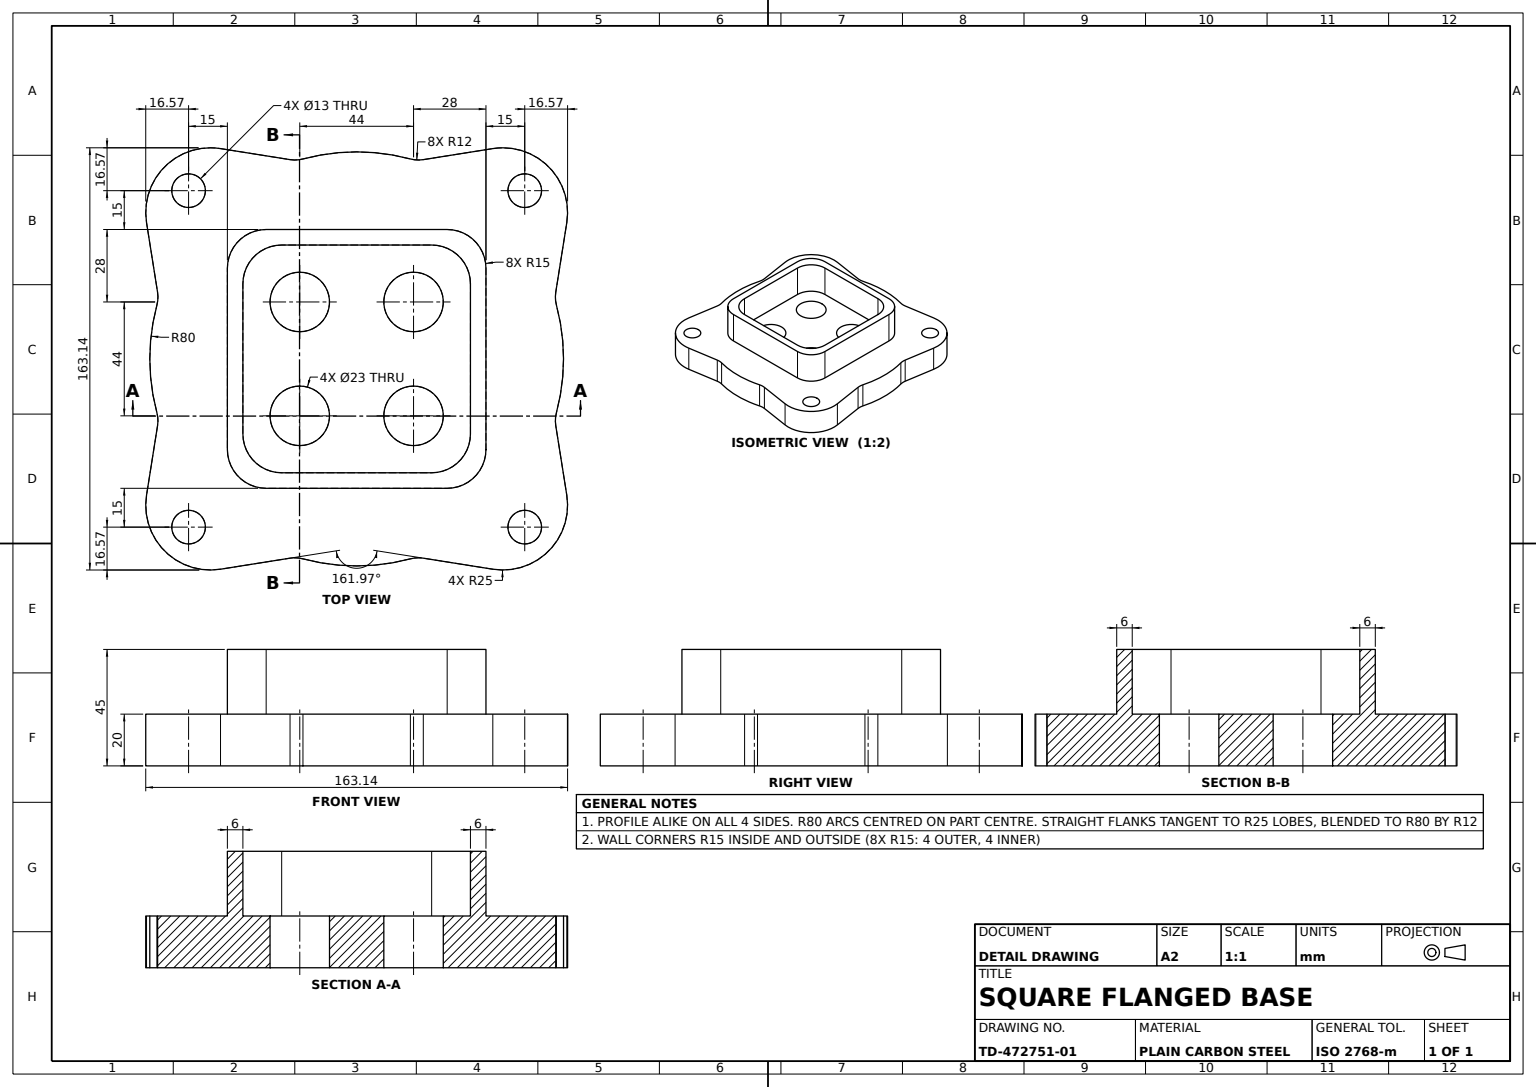
from build123d import *

# Parameters (mm, degrees)
LOBED_BASE_PLATE_DEPTH      = 20
SQUARE_POCKET_WALL_DEPTH    = 25
POCKET_HOLES_SKETCH_R       = 11.5
POCKET_FLOOR_HOLES_4X_DEPTH = 25
EDGE_FILLET_R12_A_R         = 12
EDGE_FILLET_R12_B_R         = 12
EDGE_FILLET_R12_C_R         = 12
EDGE_FILLET_R12_D_R         = 12
EDGE_FILLET_R12_E_R         = 12
EDGE_FILLET_R12_F_R         = 12
EDGE_FILLET_R12_G_R         = 12
EDGE_FILLET_R12_H_R         = 12
MOUNTING_HOLES_SKETCH_R     = 6.5
MOUNTING_HOLES_4X_DEPTH     = 25


with BuildPart() as part:
    # Lobed Base Profile → Lobed Base Plate (new body)
    with BuildSketch(Plane(origin=(0, 0, 0), x_dir=(1, 0, 0), z_dir=(0, 1, 0))):
        with BuildLine():
            Line((52.650346772, -81.259588286), (23.147950432, -76.577884476))
            ThreePointArc((23.147950432, -76.577884476), (0, -80), (-23.147950432, -76.577884476))
            Line((-23.147950432, -76.577884476), (-52.650346772, -81.259588286))
            ThreePointArc((-52.650346772, -81.259588286), (-74.246212025, -74.246212025), (-81.259588286, -52.650346772))
            Line((-81.259588286, -52.650346772), (-76.577884476, -23.147950432))
            ThreePointArc((-76.577884476, -23.147950432), (-80, 0), (-76.577884476, 23.147950432))
            Line((-76.577884476, 23.147950432), (-81.259588286, 52.650346772))
            ThreePointArc((-81.259588286, 52.650346772), (-74.246212025, 74.246212025), (-52.650346772, 81.259588286))
            Line((-52.650346772, 81.259588286), (-23.147950432, 76.577884476))
            ThreePointArc((-23.147950432, 76.577884476), (0, 80), (23.147950432, 76.577884476))
            Line((23.147950432, 76.577884476), (52.650346772, 81.259588286))
            ThreePointArc((52.650346772, 81.259588286), (74.246212025, 74.246212025), (81.259588286, 52.650346772))
            Line((81.259588286, 52.650346772), (76.577884476, 23.147950432))
            ThreePointArc((76.577884476, 23.147950432), (80, 0), (76.577884476, -23.147950432))
            Line((76.577884476, -23.147950432), (81.259588286, -52.650346772))
            ThreePointArc((81.259588286, -52.650346772), (74.246212025, -74.246212025), (52.650346772, -81.259588286))
        make_face()
    extrude(amount=LOBED_BASE_PLATE_DEPTH)

    # Square Wall Profile → Square Pocket Wall (add)
    with BuildSketch(Plane(origin=(0, 20, 0), x_dir=(1, 0, 0), z_dir=(0, 1, 0))):
        with BuildLine():
            Line((50, -1.641590962), (50, -35))
            ThreePointArc((50, -35), (45.606601718, -45.606601718), (35, -50))
            Line((35, -50), (-35, -50))
            ThreePointArc((-35, -50), (-45.606601718, -45.606601718), (-50, -35))
            Line((-50, -35), (-50, 35))
            ThreePointArc((-50, 35), (-45.606601718, 45.606601718), (-35, 50))
            Line((-35, 50), (35, 50))
            ThreePointArc((35, 50), (45.606601718, 45.606601718), (50, 35))
            Line((50, 35), (50, -1.641590962))
        make_face()
        with BuildLine():
            Line((44, -1.641590962), (44, -29))
            ThreePointArc((44, -29), (39.606601718, -39.606601718), (29, -44))
            Line((29, -44), (-29, -44))
            ThreePointArc((-29, -44), (-39.606601718, -39.606601718), (-44, -29))
            Line((-44, -29), (-44, 29))
            ThreePointArc((-44, 29), (-39.606601718, 39.606601718), (-29, 44))
            Line((-29, 44), (29, 44))
            ThreePointArc((29, 44), (39.606601718, 39.606601718), (44, 29))
            Line((44, 29), (44, -1.641590962))
        make_face(mode=Mode.SUBTRACT)
    extrude(amount=SQUARE_POCKET_WALL_DEPTH)

    # Pocket Holes Sketch → Pocket Floor Holes 4x (cut)
    with BuildSketch(Plane(origin=(0, 20, 0), x_dir=(1, 0, 0), z_dir=(0, 1, 0))):
        with Locations(Location((22, -22, 0), (0, 0, 270))):
            Circle(POCKET_HOLES_SKETCH_R)
        with Locations(Location((22, 22, 0), (0, 0, 270))):
            Circle(POCKET_HOLES_SKETCH_R)
        with Locations(Location((-22, 22, 0), (0, 0, 270))):
            Circle(POCKET_HOLES_SKETCH_R)
        with Locations(Location((-22, -22, 0), (0, 0, 270))):
            Circle(POCKET_HOLES_SKETCH_R)
    extrude(amount=-POCKET_FLOOR_HOLES_4X_DEPTH, mode=Mode.SUBTRACT)

    # Edge Fillet R12 A
    edge_fillet_r12_a_edges = [part.edges().sort_by_distance(p)[0] for p in [
        (23.147950432, 10, 76.577884476),
    ]]
    fillet(edge_fillet_r12_a_edges, radius=EDGE_FILLET_R12_A_R)

    # Edge Fillet R12 B
    edge_fillet_r12_b_edges = [part.edges().sort_by_distance(p)[0] for p in [
        (-23.147950432, 10, 76.577884476),
    ]]
    fillet(edge_fillet_r12_b_edges, radius=EDGE_FILLET_R12_B_R)

    # Edge Fillet R12 C
    edge_fillet_r12_c_edges = [part.edges().sort_by_distance(p)[0] for p in [
        (23.147950432, 10, -76.577884476),
    ]]
    fillet(edge_fillet_r12_c_edges, radius=EDGE_FILLET_R12_C_R)

    # Edge Fillet R12 D
    edge_fillet_r12_d_edges = [part.edges().sort_by_distance(p)[0] for p in [
        (-23.147950432, 10, -76.577884476),
    ]]
    fillet(edge_fillet_r12_d_edges, radius=EDGE_FILLET_R12_D_R)

    # Edge Fillet R12 E
    edge_fillet_r12_e_edges = [part.edges().sort_by_distance(p)[0] for p in [
        (76.577884476, 10, -23.147950432),
    ]]
    fillet(edge_fillet_r12_e_edges, radius=EDGE_FILLET_R12_E_R)

    # Edge Fillet R12 F
    edge_fillet_r12_f_edges = [part.edges().sort_by_distance(p)[0] for p in [
        (76.577884476, 10, 23.147950432),
    ]]
    fillet(edge_fillet_r12_f_edges, radius=EDGE_FILLET_R12_F_R)

    # Edge Fillet R12 G
    edge_fillet_r12_g_edges = [part.edges().sort_by_distance(p)[0] for p in [
        (-76.577884476, 10, 23.147950432),
    ]]
    fillet(edge_fillet_r12_g_edges, radius=EDGE_FILLET_R12_G_R)

    # Edge Fillet R12 H
    edge_fillet_r12_h_edges = [part.edges().sort_by_distance(p)[0] for p in [
        (-76.577884476, 10, -23.147950432),
    ]]
    fillet(edge_fillet_r12_h_edges, radius=EDGE_FILLET_R12_H_R)

    # Mounting Holes Sketch → Mounting Holes 4x (cut)
    with BuildSketch(Plane(origin=(0, 20, 0), x_dir=(1, 0, 0), z_dir=(0, 1, 0))):
        with Locations(Location((65, 65, 0), (0, 0, 270))):
            Circle(MOUNTING_HOLES_SKETCH_R)
        with Locations(Location((65, -65, 0), (0, 0, 270))):
            Circle(MOUNTING_HOLES_SKETCH_R)
        with Locations(Location((-65, -65, 0), (0, 0, 270))):
            Circle(MOUNTING_HOLES_SKETCH_R)
        with Locations(Location((-65, 65, 0), (0, 0, 270))):
            Circle(MOUNTING_HOLES_SKETCH_R)
    extrude(amount=-MOUNTING_HOLES_4X_DEPTH, mode=Mode.SUBTRACT)


solid = part.part
